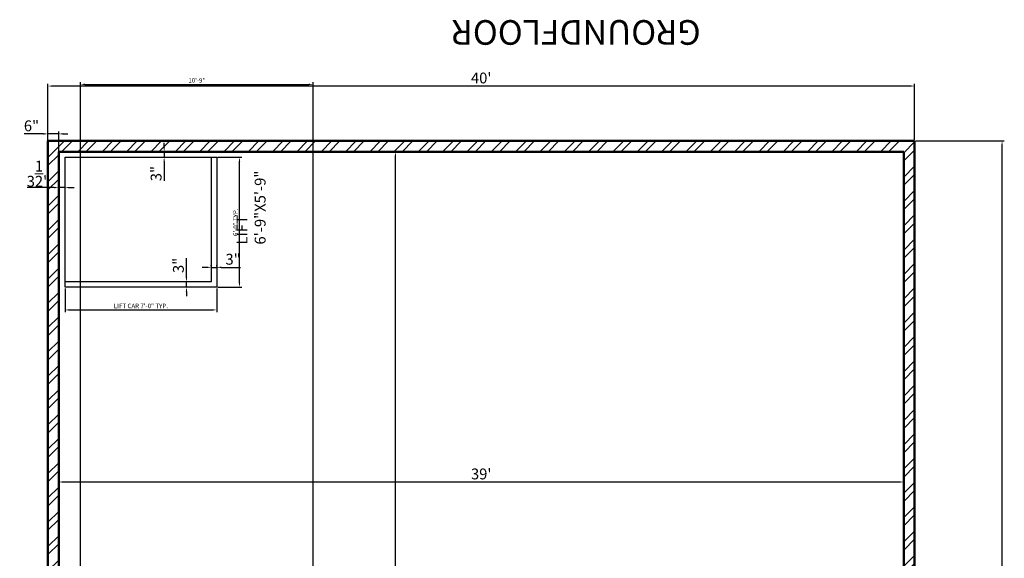
# Model space of a CAD drawing. Units: inches. Extents: x 244 to 2800, y 1060 to 1700.
# Tile 13 of 13: x 2255 to 2800, y 1402 to 1700. Entities that reach past the tile are written whole.
import ezdxf

# ---------------------------------------------------------------- set-up
doc = ezdxf.new("R2010")
doc.units = ezdxf.units.IN
for name, color, linetype, lineweight in [('A-ANNO-DIMS', 2, 'Continuous', 18), ('A-ANNO-TEXT', 1, 'Continuous', 18), ('A-EQPM', 4, 'Continuous', 25), ('A-WALL', 7, 'Continuous', 50), ('A-WALL-PATT', 8, 'Continuous', 13)]:
    doc.layers.add(name, color=color, linetype=linetype, lineweight=lineweight)
doc.styles.get("Standard").update_dxf_attribs({"font": 'arial.ttf'})
doc.dimstyles.new('ISO-25', dxfattribs={"dimtxt": 2.5, "dimasz": 2.5, "dimexe": 1.25, "dimexo": 0.625, "dimtad": 1, "dimlunit": 4, "dimtxsty": 'Standard', "dimcen": 2.5, "dimadec": 0, "dimazin": 0, "dimtfac": 1, "dimtmove": 0, "dimatfit": 3, "dimfxl": 1, "dimarcsym": 0})

# ---------------------------------------------------------------- blocks, each defined once
blk = doc.blocks.new('*D9')
at = {"layer": 'A-ANNO-DIMS', "color": 0, "lineweight": -2, "transparency": 16777216}
for p, q in [((2751.08, 1632.99), (2800.17, 1632.99)), ((2798.92, 1095.49), (2798.92, 1630.49)), ((2751.08, 1092.99), (2800.17, 1092.99))]:
    blk.add_line(p, q, dxfattribs=at)
at = {"layer": 'A-ANNO-DIMS', "color": 0, "transparency": 16777216}
for points in [[(2798.5, 1630.49), (2799.34, 1630.49), (2798.92, 1632.99)], [(2798.5, 1095.49), (2799.34, 1095.49), (2798.92, 1092.99)]]:
    blk.add_solid(points, dxfattribs=at)
at = {"layer": 'Defpoints', "color": 0, "transparency": 16777216}
for p in [(2750.46, 1632.99), (2798.92, 1632.99), (2750.46, 1092.99)]:
    blk.add_point(p, dxfattribs=at)
at = {"layer": 'A-ANNO-DIMS', "color": 0, "transparency": 16777216, "insert": (2795.24, 1362.99), "char_height": 6, "attachment_point": 5, "rotation": 90}
blk.add_mtext("45'", dxfattribs=at)
blk = doc.blocks.new('*D10')
at = {"layer": 'A-ANNO-DIMS', "color": 0, "lineweight": -2, "transparency": 16777216}
for p, q in [((2270.46, 1633.61), (2270.46, 1664.65)), ((2747.96, 1663.4), (2272.96, 1663.4)), ((2750.46, 1633.61), (2750.46, 1664.65))]:
    blk.add_line(p, q, dxfattribs=at)
at = {"layer": 'A-ANNO-DIMS', "color": 0, "transparency": 16777216}
for points in [[(2272.96, 1663.82), (2272.96, 1662.99), (2270.46, 1663.4)], [(2747.96, 1663.82), (2747.96, 1662.99), (2750.46, 1663.4)]]:
    blk.add_solid(points, dxfattribs=at)
at = {"layer": 'Defpoints', "color": 0, "transparency": 16777216}
for p in [(2270.46, 1663.4), (2270.46, 1632.99), (2750.46, 1632.99)]:
    blk.add_point(p, dxfattribs=at)
at = {"layer": 'A-ANNO-DIMS', "color": 0, "transparency": 16777216, "insert": (2510.46, 1667.09), "char_height": 6, "attachment_point": 5}
blk.add_mtext("40'", dxfattribs=at)
blk = doc.blocks.new('*D11')
at = {"layer": 'A-ANNO-DIMS', "color": 0, "lineweight": -2, "transparency": 16777216}
for p, q in [((2347.21, 1557.49), (2347.21, 1568.13)), ((2354.13, 1554.99), (2345.96, 1554.99)), ((2347.21, 1551.99), (2347.21, 1554.99)), ((2354.13, 1551.99), (2345.96, 1551.99)), ((2347.21, 1549.49), (2347.21, 1546.99))]:
    blk.add_line(p, q, dxfattribs=at)
at = {"layer": 'A-ANNO-DIMS', "color": 0, "transparency": 16777216}
for points in [[(2346.8, 1557.49), (2347.63, 1557.49), (2347.21, 1554.99)], [(2346.8, 1549.49), (2347.63, 1549.49), (2347.21, 1551.99)]]:
    blk.add_solid(points, dxfattribs=at)
at = {"layer": 'Defpoints', "color": 0, "transparency": 16777216}
for p in [(2347.21, 1554.99), (2354.76, 1554.99), (2354.76, 1551.99)]:
    blk.add_point(p, dxfattribs=at)
at = {"layer": 'A-ANNO-DIMS', "color": 0, "transparency": 16777216, "insert": (2343.52, 1564.06), "char_height": 6, "attachment_point": 5, "rotation": 90}
blk.add_mtext('3"', dxfattribs=at)
blk = doc.blocks.new('*D12')
at = {"layer": 'A-ANNO-DIMS', "color": 0, "lineweight": -2, "transparency": 16777216}
for p, q in [((2358.47, 1562.99), (2355.97, 1562.99)), ((2360.97, 1563.62), (2360.97, 1564.24)), ((2360.97, 1562.99), (2363.97, 1562.99)), ((2363.97, 1563.62), (2363.97, 1564.24)), ((2366.47, 1562.99), (2377.11, 1562.99))]:
    blk.add_line(p, q, dxfattribs=at)
at = {"layer": 'A-ANNO-DIMS', "color": 0, "transparency": 16777216}
for points in [[(2358.47, 1563.41), (2358.47, 1562.58), (2360.97, 1562.99)], [(2366.47, 1563.41), (2366.47, 1562.58), (2363.97, 1562.99)]]:
    blk.add_solid(points, dxfattribs=at)
at = {"layer": 'Defpoints', "color": 0, "transparency": 16777216}
for p in [(2360.97, 1562.99), (2363.97, 1562.99), (2363.97, 1562.99)]:
    blk.add_point(p, dxfattribs=at)
at = {"layer": 'A-ANNO-DIMS', "color": 0, "transparency": 16777216, "insert": (2373.04, 1566.68), "char_height": 6, "attachment_point": 5}
blk.add_mtext('3"', dxfattribs=at)
blk = doc.blocks.new('*D13')
at = {"layer": 'A-ANNO-DIMS', "color": 0, "lineweight": -2, "transparency": 16777216}
for p, q in [((2334.85, 1629.49), (2334.85, 1631.99)), ((2334.85, 1626.99), (2334.85, 1623.99)), ((2335.48, 1626.99), (2336.1, 1626.99)), ((2334.85, 1621.49), (2334.85, 1610.84)), ((2335.48, 1623.99), (2336.1, 1623.99))]:
    blk.add_line(p, q, dxfattribs=at)
at = {"layer": 'A-ANNO-DIMS', "color": 0, "transparency": 16777216}
for points in [[(2334.44, 1629.49), (2335.27, 1629.49), (2334.85, 1626.99)], [(2334.44, 1621.49), (2335.27, 1621.49), (2334.85, 1623.99)]]:
    blk.add_solid(points, dxfattribs=at)
at = {"layer": 'Defpoints', "color": 0, "transparency": 16777216}
for p in [(2334.85, 1626.99), (2334.85, 1623.99), (2334.85, 1623.99)]:
    blk.add_point(p, dxfattribs=at)
at = {"layer": 'A-ANNO-DIMS', "color": 0, "transparency": 16777216, "insert": (2331.16, 1614.92), "char_height": 6, "attachment_point": 5, "rotation": 90}
blk.add_mtext('3"', dxfattribs=at)
blk = doc.blocks.new('*D14')
at = {"layer": 'A-ANNO-DIMS', "color": 0, "lineweight": -2, "transparency": 16777216}
for p, q in [((2273.96, 1607.15), (2258.94, 1607.15)), ((2276.46, 1605.32), (2276.46, 1608.4)), ((2279.97, 1607.15), (2276.46, 1607.15)), ((2279.97, 1605.32), (2279.97, 1608.4)), ((2282.47, 1607.15), (2284.97, 1607.15))]:
    blk.add_line(p, q, dxfattribs=at)
at = {"layer": 'A-ANNO-DIMS', "color": 0, "transparency": 16777216}
for points in [[(2273.96, 1607.57), (2273.96, 1606.74), (2276.46, 1607.15)], [(2282.47, 1607.57), (2282.47, 1606.74), (2279.97, 1607.15)]]:
    blk.add_solid(points, dxfattribs=at)
at = {"layer": 'Defpoints', "color": 0, "transparency": 16777216}
for p in [(2276.46, 1607.15), (2276.46, 1604.69), (2279.97, 1604.69)]:
    blk.add_point(p, dxfattribs=at)
at = {"layer": 'A-ANNO-DIMS', "color": 0, "transparency": 16777216, "insert": (2265.2, 1614.86), "char_height": 6, "attachment_point": 5}
blk.add_mtext('3{\\H1x;\\S1/2;}"', dxfattribs=at)
blk = doc.blocks.new('*D17')
at = {"layer": 'A-ANNO-DIMS', "color": 0, "lineweight": -2, "transparency": 16777216}
for p, q in [((2267.96, 1636.9), (2257.28, 1636.9)), ((2270.46, 1623.68), (2270.46, 1638.15)), ((2276.46, 1636.9), (2270.46, 1636.9)), ((2276.46, 1623.68), (2276.46, 1638.15)), ((2278.96, 1636.9), (2281.46, 1636.9))]:
    blk.add_line(p, q, dxfattribs=at)
at = {"layer": 'A-ANNO-DIMS', "color": 0, "transparency": 16777216}
for points in [[(2267.96, 1637.32), (2267.96, 1636.49), (2270.46, 1636.9)], [(2278.96, 1637.32), (2278.96, 1636.49), (2276.46, 1636.9)]]:
    blk.add_solid(points, dxfattribs=at)
at = {"layer": 'Defpoints', "color": 0, "transparency": 16777216}
for p in [(2270.46, 1636.9), (2270.46, 1623.06), (2276.46, 1623.06)]:
    blk.add_point(p, dxfattribs=at)
at = {"layer": 'A-ANNO-DIMS', "color": 0, "transparency": 16777216, "insert": (2261.37, 1640.59), "char_height": 6, "attachment_point": 5}
blk.add_mtext('6"', dxfattribs=at)
blk = doc.blocks.new('*D44')
at = {"layer": 'A-ANNO-DIMS', "color": 0, "lineweight": -2, "transparency": 16777216}
for p, q in [((2276.46, 1405.21), (2276.46, 1445.34)), ((2744.46, 1405.21), (2744.46, 1445.34)), ((2741.96, 1444.09), (2278.96, 1444.09))]:
    blk.add_line(p, q, dxfattribs=at)
at = {"layer": 'A-ANNO-DIMS', "color": 0, "transparency": 16777216}
for points in [[(2278.96, 1444.51), (2278.96, 1443.67), (2276.46, 1444.09)], [(2741.96, 1444.51), (2741.96, 1443.67), (2744.46, 1444.09)]]:
    blk.add_solid(points, dxfattribs=at)
at = {"layer": 'Defpoints', "color": 0, "transparency": 16777216}
for p in [(2276.46, 1444.09), (2276.46, 1404.59), (2744.46, 1404.59)]:
    blk.add_point(p, dxfattribs=at)
at = {"layer": 'A-ANNO-DIMS', "color": 0, "transparency": 16777216, "insert": (2510.46, 1447.78), "char_height": 6, "attachment_point": 5}
blk.add_mtext("39'", dxfattribs=at)
blk = doc.blocks.new('*D45')
at = {"layer": 'A-ANNO-DIMS', "color": 0, "lineweight": -2, "transparency": 16777216}
for p, q in [((2478.2, 1626.99), (2461.68, 1626.99)), ((2462.93, 1101.49), (2462.93, 1624.49)), ((2478.2, 1098.99), (2461.68, 1098.99))]:
    blk.add_line(p, q, dxfattribs=at)
at = {"layer": 'A-ANNO-DIMS', "color": 0, "transparency": 16777216}
for points in [[(2462.51, 1624.49), (2463.34, 1624.49), (2462.93, 1626.99)], [(2462.51, 1101.49), (2463.34, 1101.49), (2462.93, 1098.99)]]:
    blk.add_solid(points, dxfattribs=at)
at = {"layer": 'Defpoints', "color": 0, "transparency": 16777216}
for p in [(2462.93, 1626.99), (2478.82, 1626.99), (2478.82, 1098.99)]:
    blk.add_point(p, dxfattribs=at)
at = {"layer": 'A-ANNO-DIMS', "color": 0, "transparency": 16777216, "insert": (2459.3, 1362.99), "char_height": 6, "attachment_point": 5, "rotation": 90}
blk.add_mtext("44'", dxfattribs=at)
blk = doc.blocks.new('LIFT-CAR')
for p, q in [((0, 0), (0, 72)), ((0, 72), (84, 72)), ((81, 72), (81, 3)), ((84, 72), (84, 0)), ((81, 3), (0, 3)), ((84, 0), (0, 0))]:
    blk.add_line(p, q)
blk = doc.blocks.new('*D64')
at = {"layer": 'A-ANNO-DIMS', "color": 0, "lineweight": -2, "transparency": 16777216}
for p, q in [((2279.97, 1551.36), (2279.97, 1538.14)), ((2363.97, 1551.36), (2363.97, 1538.14)), ((2282.47, 1539.39), (2361.47, 1539.39))]:
    blk.add_line(p, q, dxfattribs=at)
at = {"layer": 'A-ANNO-DIMS', "color": 0, "transparency": 16777216}
for points in [[(2282.47, 1539.8), (2282.47, 1538.97), (2279.97, 1539.39)], [(2361.47, 1539.8), (2361.47, 1538.97), (2363.97, 1539.39)]]:
    blk.add_solid(points, dxfattribs=at)
at = {"layer": 'Defpoints', "color": 0, "transparency": 16777216}
for p in [(2279.97, 1551.99), (2363.97, 1551.99), (2363.97, 1539.39)]:
    blk.add_point(p, dxfattribs=at)
at = {"layer": 'A-ANNO-DIMS', "color": 0, "transparency": 16777216, "insert": (2321.97, 1541.3), "char_height": 2.5, "attachment_point": 5}
blk.add_mtext('LIFT CAR 7\'-0" TYP.', dxfattribs=at)
blk = doc.blocks.new('*D65')
at = {"layer": 'A-ANNO-DIMS', "color": 0, "lineweight": -2, "transparency": 16777216}
for p, q in [((2364.6, 1623.99), (2377.82, 1623.99)), ((2376.57, 1554.49), (2376.57, 1621.49)), ((2364.6, 1551.99), (2377.82, 1551.99))]:
    blk.add_line(p, q, dxfattribs=at)
at = {"layer": 'A-ANNO-DIMS', "color": 0, "transparency": 16777216}
for points in [[(2376.16, 1621.49), (2376.99, 1621.49), (2376.57, 1623.99)], [(2376.16, 1554.49), (2376.99, 1554.49), (2376.57, 1551.99)]]:
    blk.add_solid(points, dxfattribs=at)
at = {"layer": 'Defpoints', "color": 0, "transparency": 16777216}
for p in [(2363.97, 1623.99), (2376.57, 1623.99), (2363.97, 1551.99)]:
    blk.add_point(p, dxfattribs=at)
at = {"layer": 'A-ANNO-DIMS', "color": 0, "transparency": 16777216, "insert": (2374.67, 1587.99), "char_height": 2.5, "attachment_point": 5, "rotation": 90}
blk.add_mtext('6\'-0" TYP.', dxfattribs=at)
blk = doc.blocks.new('*D148')
at = {"layer": 'A-ANNO-DIMS', "color": 0, "lineweight": -2, "transparency": 16777216}
for p, q in [((2288.46, 1289.61), (2288.46, 1665.59)), ((2290.96, 1664.34), (2414.96, 1664.34)), ((2417.46, 1289.61), (2417.46, 1665.59))]:
    blk.add_line(p, q, dxfattribs=at)
at = {"layer": 'A-ANNO-DIMS', "color": 0, "transparency": 16777216}
for points in [[(2290.96, 1664.75), (2290.96, 1663.92), (2288.46, 1664.34)], [(2414.96, 1664.75), (2414.96, 1663.92), (2417.46, 1664.34)]]:
    blk.add_solid(points, dxfattribs=at)
at = {"layer": 'Defpoints', "color": 0, "transparency": 16777216}
for p in [(2417.46, 1664.34), (2288.46, 1288.99), (2417.46, 1288.99)]:
    blk.add_point(p, dxfattribs=at)
at = {"layer": 'A-ANNO-DIMS', "color": 0, "transparency": 16777216, "insert": (2352.96, 1666.24), "char_height": 2.5, "attachment_point": 5}
blk.add_mtext('10\'-9"', dxfattribs=at)

msp = doc.modelspace()

# ---------------------------------------------------------------- hatches: boundary and pattern name
at = {"layer": 'A-WALL-PATT'}
h = msp.add_hatch(dxfattribs=at)
h.set_pattern_fill('ANSI32', color=256)
h.paths.add_polyline_path([(2750.457, 1632.986), (2270.457, 1632.986), (2270.457, 1092.986), (2750.457, 1092.986)])
h.paths.add_polyline_path([(2276.457, 1626.986), (2744.457, 1626.986), (2744.457, 1098.986), (2660.457, 1098.986), (2276.457, 1098.986)], flags=16)
h.paths.add_polyline_path([(2288.457, 1288.986), (2417.457, 1288.986), (2417.457, 1281.486), (2412.957, 1281.486), (2412.957, 1284.486), (2292.957, 1284.486), (2292.957, 1164.486), (2412.957, 1164.486), (2412.957, 1239.486), (2417.457, 1239.486), (2417.457, 1161.986), (2379.957, 1161.986), (2379.957, 1158.986), (2376.957, 1158.986), (2376.957, 1161.986), (2292.957, 1161.986), (2292.957, 1113.986), (2376.957, 1113.986), (2376.957, 1128.986), (2379.957, 1128.986), (2379.957, 1110.986), (2288.457, 1110.986)], flags=0)
h.paths.add_polyline_path([(2288.457, 1279.202), (2292.957, 1279.202), (2292.957, 1243.232), (2288.457, 1243.232)], flags=0)
h.paths.add_polyline_path([(2290.907, 1278.702), (2290.907, 1243.732), (2290.507, 1243.732), (2290.507, 1278.702)], flags=0)
h.paths.add_polyline_path([(2288.457, 1151.417), (2292.957, 1151.417), (2292.957, 1127.404), (2288.457, 1127.404)], flags=0)
h.paths.add_polyline_path([(2290.907, 1150.917), (2290.907, 1127.904), (2290.507, 1127.904), (2290.507, 1150.917)], flags=0)
h.paths.add_polyline_path([(2279.972, 1551.986), (2279.972, 1623.986), (2363.972, 1623.986), (2363.972, 1551.986)], flags=0)
h.paths.add_polyline_path([(2660.457, 1242.986), (2696.457, 1242.986), (2696.457, 1134.986), (2708.457, 1134.986), (2708.457, 1242.986), (2744.457, 1242.986), (2744.457, 1134.986), (2660.457, 1134.986)], flags=0)
h.paths.add_polyline_path([(2379.957, 1128.986), (2376.957, 1128.986), (2376.957, 1113.986), (2292.957, 1113.986), (2292.957, 1127.404), (2288.457, 1127.404), (2288.457, 1110.986), (2379.957, 1110.986)], flags=0)
h.paths.add_polyline_path([(2417.457, 1239.486), (2412.957, 1239.486), (2412.957, 1164.486), (2292.957, 1164.486), (2292.957, 1161.986), (2376.957, 1161.986), (2417.457, 1161.986)], flags=0)
h.paths.add_polyline_path([(2289.96, 1267.789), (2275.356, 1267.789), (2275.356, 1256.194), (2289.96, 1256.194)], flags=24)
h.paths.add_polyline_path([(2289.96, 1145.072), (2275.356, 1145.072), (2275.356, 1133.477), (2289.96, 1133.477)], flags=24)
h.paths.add_polyline_path([(2406.937, 1224.517), (2290.255, 1224.517), (2290.255, 1173.588), (2406.937, 1173.588)], flags=8)
h.paths.add_polyline_path([(2351.026, 1148.815), (2293.304, 1148.815), (2293.304, 1118.024), (2351.026, 1118.024)], flags=8)
h.paths.add_polyline_path([(2383.007, 1159.633), (2352.857, 1159.633), (2352.857, 1132.452), (2383.007, 1132.452)], flags=8)
h.paths.add_polyline_path([(2421.657, 1275.631), (2391.507, 1275.631), (2391.507, 1248.45), (2421.657, 1248.45)], flags=8)
h.paths.add_polyline_path([(2394.334, 1573.477), (2394.334, 1615.869), (2371.88, 1615.869), (2371.88, 1573.477)], flags=8)
h.paths.add_polyline_path([(2726.202, 1266.003), (2669.205, 1266.003), (2669.205, 1252.05), (2726.202, 1252.05)], flags=8)

# ---------------------------------------------------------------- linework, layer by layer
at = {"layer": 'A-WALL'}
for p, q in [((2750.457, 1632.986), (2270.457, 1632.986)), ((2270.457, 1632.986), (2270.457, 1092.986)), ((2750.457, 1092.986), (2750.457, 1632.986)), ((2744.457, 1626.986), (2276.457, 1626.986)), ((2276.457, 1626.986), (2276.457, 1098.986)), ((2744.457, 1098.986), (2744.457, 1626.986))]:
    msp.add_line(p, q, dxfattribs=at)

# ---------------------------------------------------------------- block references
at = {"layer": 'A-EQPM'}
msp.add_blockref('LIFT-CAR', (2279.972, 1551.986), dxfattribs=at)

# ---------------------------------------------------------------- texts
at = {"layer": 'A-ANNO-TEXT', "attachment_point": 1}
for s, width, gutter_width, insert, char_height, rotation in [('GROUNDFLOOR', 25.27039, 68.243, (2632.012, 1686.264), 13.64851, 180), ('LIFT\\P6\'-9"X5\'-9"', 12.02436, 30.086, (2374.977, 1575.597), 6.01727, 90)]:
    msp.add_mtext_dynamic_manual_height_columns(s, width=width, gutter_width=gutter_width, heights=[0], dxfattribs=dict(at, insert=insert, char_height=char_height, rotation=rotation))

# ---------------------------------------------------------------- dimensions: what is measured, and where the dimension line sits
at = {"layer": 'A-ANNO-DIMS'}
for base, p1, p2, override, picture, middle in [((2270.457, 1663.405), (2750.457, 1632.986), (2270.457, 1632.986), {"dimtxt": 6, "dimclrd": 0, "dimclre": 0, "dimclrt": 0}, '*D10', (2510.457, 1667.093)), ((2417.457, 1664.336), (2288.457, 1288.986), (2417.457, 1288.986), {"dimdec": 1, "dimlfac": 1, "dimrnd": 0, "dimzin": 1, "dimdsep": 46, "dimlunit": 4, "dimfrac": 2}, '*D148', (2352.957, 1666.238)), ((2270.457, 1636.902), (2276.457, 1623.058), (2270.457, 1623.058), {"dimtxt": 6, "dimclrd": 0, "dimclre": 0, "dimclrt": 0}, '*D17', (2261.367, 1640.59)), ((2276.457, 1607.1541), (2279.9718, 1604.6934), (2276.457, 1604.6934), {"dimtxt": 6, "dimclrd": 0, "dimclre": 0, "dimclrt": 0}, '*D14', (2265.1983, 1614.8569)), ((2363.972, 1562.992), (2360.972, 1562.992), (2363.972, 1562.992), {"dimtxt": 6, "dimclrd": 0, "dimclre": 0, "dimclrt": 0}, '*D12', (2373.043, 1566.683)), ((2276.457, 1444.091), (2744.457, 1404.588), (2276.457, 1404.588), {"dimtxt": 6, "dimclrd": 0, "dimclre": 0, "dimclrt": 0}, '*D44', (2510.457, 1447.781))]:
    dim = msp.add_linear_dim(base=base, p1=p1, p2=p2, dimstyle='ISO-25', override=override, dxfattribs=at)
    dim.commit()
    dim.dimension.update_dxf_attribs({"geometry": picture, "text_midpoint": middle})
for base, p1, p2, picture, middle in [((2334.854, 1623.986), (2334.854, 1626.986), (2334.854, 1623.986), '*D13', (2331.164, 1614.915)), ((2798.92, 1632.986), (2750.457, 1092.986), (2750.457, 1632.986), '*D9', (2795.244, 1362.986)), ((2462.925, 1626.986), (2478.822, 1098.986), (2478.822, 1626.986), '*D45', (2459.3, 1362.986)), ((2347.212, 1554.986), (2354.756, 1551.986), (2354.756, 1554.986), '*D11', (2343.522, 1564.057))]:
    dim = msp.add_linear_dim(base=base, p1=p1, p2=p2, angle=90, dimstyle='ISO-25', override={"dimtxt": 6, "dimclrd": 0, "dimclre": 0, "dimclrt": 0}, dxfattribs=at)
    dim.commit()
    dim.dimension.update_dxf_attribs({"geometry": picture, "text_midpoint": middle})
dim = msp.add_linear_dim(base=(2376.572, 1623.986), p1=(2363.972, 1551.986), p2=(2363.972, 1623.986), angle=90, text='<> TYP.', dimstyle='ISO-25', override={"dimdec": 1, "dimrnd": 0, "dimzin": 1, "dimlunit": 4, "dimfrac": 2}, dxfattribs=at)
dim.commit()
dim.dimension.update_dxf_attribs({"geometry": '*D65', "text_midpoint": (2374.67, 1587.986)})
dim = msp.add_linear_dim(base=(2363.972, 1539.386), p1=(2279.972, 1551.986), p2=(2363.972, 1551.986), text='LIFT CAR <> TYP.', dimstyle='ISO-25', override={"dimdec": 1, "dimrnd": 0, "dimzin": 1, "dimlunit": 4, "dimfrac": 2}, dxfattribs=at)
dim.commit()
dim.dimension.update_dxf_attribs({"geometry": '*D64', "text_midpoint": (2321.972, 1541.304)})

doc.saveas('drawing.dxf')
